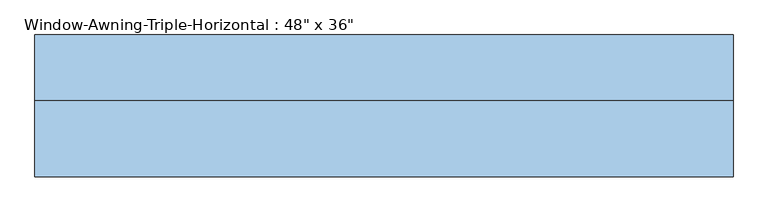
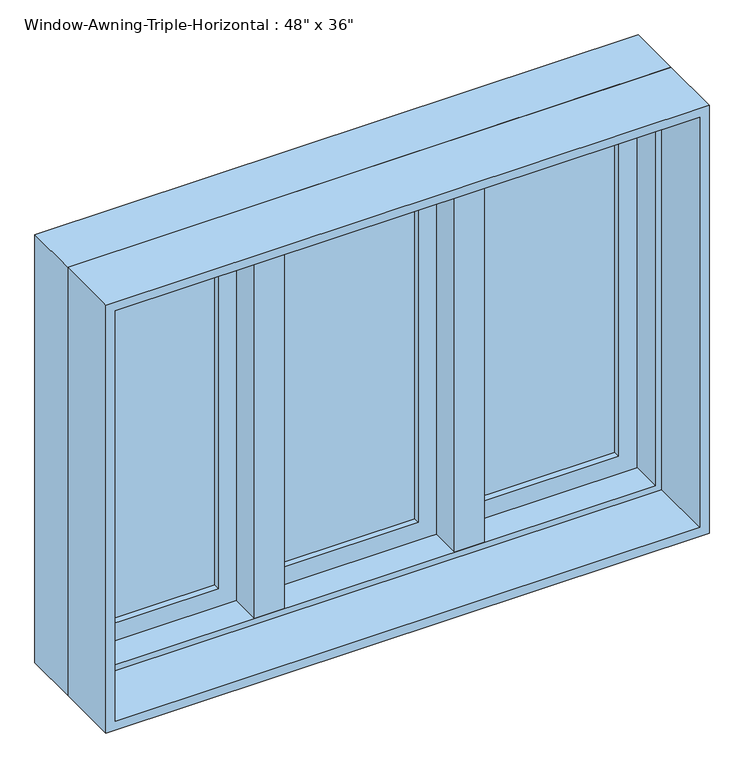
"""IFC4 building model written with IfcOpenShell, lengths in millimetres: window geometry."""

from ifc_helpers import new_model, si_unit, frame, origin, place, context, project, spatial, polyline, outline, extrude, faceted_brep, source, transform, mapped, element, save


def window_06177765(model_context):
    return source(origin(), model_context, "Body", "SolidModel", [
        faceted_brep([(577.85, 82.55, 1797.05), (577.85, 19.05, 1797.05), (-577.85, 19.05, 1797.05), (-577.85, 82.55, 1797.05), (596.9, 133.35, 1816.1), (596.9, 82.55, 1816.1), (-596.9, 82.55, 1816.1), (-596.9, 133.35, 1816.1), (609.6, 19.05, 1828.8), (609.6, 133.35, 1828.8), (-609.6, 133.35, 1828.8), (-609.6, 19.05, 1828.8), (-577.85, 19.05, 946.15), (-577.85, 82.55, 946.15), (-596.9, 82.55, 927.1), (-596.9, 133.35, 927.1), (-609.6, 133.35, 914.4), (-609.6, 19.05, 914.4), (577.85, 19.05, 946.15), (577.85, 82.55, 946.15), (596.9, 82.55, 927.1), (596.9, 133.35, 927.1), (609.6, 133.35, 914.4), (609.6, 19.05, 914.4)], [[[0, 1, 2, 3]], [[4, 5, 6, 7]], [[8, 9, 10, 11]], [[3, 2, 12, 13]], [[7, 6, 14, 15]], [[11, 10, 16, 17]], [[13, 12, 18, 19]], [[15, 14, 20, 21]], [[17, 16, 22, 23]], [[11, 17, 23, 8], [1, 18, 12, 2]], [[19, 18, 1, 0]], [[5, 20, 14, 6], [3, 13, 19, 0]], [[21, 20, 5, 4]], [[23, 22, 9, 8]], [[9, 22, 16, 10], [7, 15, 21, 4]]]),
        extrude(outline(polyline([(1828.8, -609.6), (914.4, -609.6), (914.4, 609.6), (1828.8, 609.6), (1828.8, -609.6)]), holes=[polyline([(1809.75, 590.55), (933.45, 590.55), (933.45, -590.55), (1809.75, -590.55), (1809.75, 590.55)])]), frame((0.0, -114.3, 0.0), z_axis=(0.0, 1.0, 0.0), x_axis=(0.0, 0.0, 1.0)), (0.0, 0.0, 1.0), 133.35),
        extrude(outline(polyline([(927.1, 596.9), (1816.1, 596.9), (1816.1, 211.6666667), (927.1, 211.6666667), (927.1, 596.9)]), holes=[polyline([(984.25, 268.8166667), (1758.95, 268.8166667), (1758.95, 539.75), (984.25, 539.75), (984.25, 268.8166667)])]), frame((0.0, 82.55, 0.0), z_axis=(0.0, 1.0, 0.0), x_axis=(0.0, 0.0, 1.0)), (0.0, 0.0, 1.0), 44.45),
        extrude(outline(polyline([(1816.1, -596.9), (927.1, -596.9), (927.1, -211.6666667), (1816.1, -211.6666667), (1816.1, -596.9)]), holes=[polyline([(1758.95, -268.8166667), (984.25, -268.8166667), (984.25, -539.75), (1758.95, -539.75), (1758.95, -268.8166667)])]), frame((0.0, 82.55, 0.0), z_axis=(0.0, 1.0, 0.0), x_axis=(0.0, 0.0, 1.0)), (0.0, 0.0, 1.0), 44.45),
        extrude(outline(polyline([(539.75, 114.3), (539.75, 107.95), (268.8166667, 107.95), (268.8166667, 114.3), (539.75, 114.3)])), frame((0.0, 0.0, 984.25), z_axis=(0.0, 0.0, 1.0), x_axis=(1.0, 0.0, 0.0)), (0.0, 0.0, 1.0), 774.7),
        extrude(outline(polyline([(268.8166667, 95.25), (268.8166667, 101.6), (539.75, 101.6), (539.75, 95.25), (268.8166667, 95.25)])), frame((0.0, 0.0, 984.25), z_axis=(0.0, 0.0, 1.0), x_axis=(1.0, 0.0, 0.0)), (0.0, 0.0, 1.0), 774.7),
        extrude(outline(polyline([(-268.8166667, 114.3), (-268.8166667, 107.95), (-539.75, 107.95), (-539.75, 114.3), (-268.8166667, 114.3)])), frame((0.0, 0.0, 984.25), z_axis=(0.0, 0.0, 1.0), x_axis=(1.0, 0.0, 0.0)), (0.0, 0.0, 1.0), 774.7),
        extrude(outline(polyline([(-539.75, 95.25), (-539.75, 101.6), (-268.8166667, 101.6), (-268.8166667, 95.25), (-539.75, 95.25)])), frame((0.0, 0.0, 984.25), z_axis=(0.0, 0.0, 1.0), x_axis=(1.0, 0.0, 0.0)), (0.0, 0.0, 1.0), 774.7),
        extrude(outline(polyline([(135.4666667, 114.3), (135.4666667, 107.95), (-135.4666667, 107.95), (-135.4666667, 114.3), (135.4666667, 114.3)])), frame((0.0, 0.0, 984.25), z_axis=(0.0, 0.0, 1.0), x_axis=(1.0, 0.0, 0.0)), (0.0, 0.0, 1.0), 774.7),
        extrude(outline(polyline([(-135.4666667, 95.25), (-135.4666667, 101.6), (135.4666667, 101.6), (135.4666667, 95.25), (-135.4666667, 95.25)])), frame((0.0, 0.0, 984.25), z_axis=(0.0, 0.0, 1.0), x_axis=(1.0, 0.0, 0.0)), (0.0, 0.0, 1.0), 774.7),
        extrude(outline(polyline([(927.1, 192.6166667), (1816.1, 192.6166667), (1816.1, -192.6166667), (927.1, -192.6166667), (927.1, 192.6166667)]), holes=[polyline([(984.25, -135.4666667), (1758.95, -135.4666667), (1758.95, 135.4666667), (984.25, 135.4666667), (984.25, -135.4666667)])]), frame((0.0, 82.55, 0.0), z_axis=(0.0, 1.0, 0.0), x_axis=(0.0, 0.0, 1.0)), (0.0, 0.0, 1.0), 44.45),
        faceted_brep([(192.6166667, 82.55, 1816.1), (172.1065328, 82.55, 1816.1), (172.1065328, 19.05, 1816.1), (232.1768005, 19.05, 1816.1), (232.1768005, 82.55, 1816.1), (211.6666667, 82.55, 1816.1), (211.6666667, 133.35, 1816.1), (192.6166667, 133.35, 1816.1), (192.6166667, 133.35, 927.1), (211.6666667, 133.35, 927.1), (211.6666667, 104.775, 927.1), (192.6166667, 104.775, 927.1), (192.6166667, 82.55, 1809.75), (172.1065328, 82.55, 1809.75), (192.6166667, 82.55, 1797.05), (192.6166667, 82.55, 946.15), (172.1065328, 82.55, 946.15), (172.1065328, 82.55, 1797.05), (172.1065328, 19.05, 1809.75), (172.1065328, 19.05, 946.15), (172.1065328, 19.05, 1797.05), (232.1768005, 19.05, 1809.75), (232.1768005, 19.05, 946.15), (232.1768005, 19.05, 1797.05), (232.1768005, 82.55, 1809.75), (232.1768005, 82.55, 946.15), (232.1768005, 82.55, 1797.05), (211.6666667, 82.55, 1809.75), (211.6666667, 82.55, 946.15), (211.6666667, 82.55, 1797.05), (211.6666667, 104.775, 1809.75), (211.6666667, 104.775, 1797.05), (211.6666667, 104.775, 946.15), (192.6166667, 104.775, 946.15), (192.6166667, 104.775, 1797.05), (192.6166667, 104.775, 1809.75)], [[[0, 1, 2, 3, 4, 5, 6, 7]], [[8, 9, 10, 11]], [[1, 0, 12, 13]], [[14, 15, 16, 17]], [[2, 1, 13, 18]], [[17, 16, 19, 20]], [[3, 2, 18, 21]], [[20, 19, 22, 23]], [[4, 3, 21, 24]], [[23, 22, 25, 26]], [[5, 4, 24, 27]], [[26, 25, 28, 29]], [[6, 5, 27, 30, 31, 29, 28, 32, 10, 9]], [[0, 7, 8, 11, 33, 15, 14, 34, 35, 12]], [[30, 35, 34, 31]], [[32, 33, 11, 10]], [[35, 30, 27, 24, 21, 18, 13, 12]], [[31, 34, 14, 17, 20, 23, 26, 29]], [[33, 32, 28, 25, 22, 19, 16, 15]], [[7, 6, 9, 8]]]),
        faceted_brep([(-211.6666667, 82.55, 1816.1), (-232.1768005, 82.55, 1816.1), (-232.1768005, 19.05, 1816.1), (-172.1065328, 19.05, 1816.1), (-172.1065328, 82.55, 1816.1), (-192.6166667, 82.55, 1816.1), (-192.6166667, 133.35, 1816.1), (-211.6666667, 133.35, 1816.1), (-211.6666667, 133.35, 927.1), (-192.6166667, 133.35, 927.1), (-192.6166667, 104.775, 927.1), (-211.6666667, 104.775, 927.1), (-232.1768005, 82.55, 1809.75), (-232.1768005, 19.05, 1809.75), (-232.1768005, 82.55, 1797.05), (-232.1768005, 82.55, 946.15), (-232.1768005, 19.05, 946.15), (-232.1768005, 19.05, 1797.05), (-172.1065328, 19.05, 1809.75), (-172.1065328, 19.05, 946.15), (-172.1065328, 19.05, 1797.05), (-172.1065328, 82.55, 1809.75), (-172.1065328, 82.55, 946.15), (-172.1065328, 82.55, 1797.05), (-192.6166667, 82.55, 1809.75), (-192.6166667, 104.775, 1809.75), (-192.6166667, 104.775, 1797.05), (-192.6166667, 82.55, 1797.05), (-192.6166667, 82.55, 946.15), (-192.6166667, 104.775, 946.15), (-211.6666667, 104.775, 946.15), (-211.6666667, 82.55, 946.15), (-211.6666667, 82.55, 1797.05), (-211.6666667, 104.775, 1797.05), (-211.6666667, 104.775, 1809.75), (-211.6666667, 82.55, 1809.75)], [[[0, 1, 2, 3, 4, 5, 6, 7]], [[8, 9, 10, 11]], [[2, 1, 12, 13]], [[14, 15, 16, 17]], [[3, 2, 13, 18]], [[17, 16, 19, 20]], [[4, 3, 18, 21]], [[20, 19, 22, 23]], [[6, 5, 24, 25, 26, 27, 28, 29, 10, 9]], [[0, 7, 8, 11, 30, 31, 32, 33, 34, 35]], [[25, 34, 33, 26]], [[29, 30, 11, 10]], [[34, 25, 24, 21, 18, 13, 12, 35]], [[26, 33, 32, 14, 17, 20, 23, 27]], [[30, 29, 28, 22, 19, 16, 15, 31]], [[1, 0, 35, 12]], [[15, 14, 32, 31]], [[5, 4, 21, 24]], [[28, 27, 23, 22]], [[7, 6, 9, 8]]]),
    ])


if __name__ == "__main__":
    model = new_model("IFC4")
    model_context = context("Model", 3, world=origin())
    ifc_project = project(units=[si_unit("LENGTHUNIT", "METRE", prefix="MILLI")], contexts=[model_context])
    site = spatial("IfcSite", under=ifc_project)
    building = spatial("IfcBuilding", under=site)
    placement = place(None, origin())
    window_shape = window_06177765(model_context)
    element("IfcWindow", 1, ObjectType="Window-Awning-Triple-Horizontal : 48\" x 36\"", at=placement, inside=building, context=model_context, shape_type="MappedRepresentation", body=[
        mapped(window_shape, transform((0.0, 0.0, 0.0), x_axis=(1.0, 0.0, 0.0), y_axis=(0.0, 1.0, 0.0), z_axis=(0.0, 0.0, 1.0))),
    ])
    save(model, "model.ifc")

# Revit data of these elements
# Type "Window-Awning-Triple-Horizontal : 48\" x 36\""
#   Type Mark = "24"
#   Fire Rating = "0.5h"
#   Analytic Construction = "Double glazing - domestic"
#   Window Inset [instance default] = 0' - 0"
#   Wall Thickness [instance default] = 0' - 6"
#   Muntin Width = 0' - 10.66667"
#   Visual Light Transmittance = 0.81
#   Thermal Resistance (R) = 1.8146 (h·ft²·°F)/BTU
#   Solar Heat Gain Coefficient = 0.76
#   One Third Width = 1' - 4"
#   Sash Width = 1' - 3.16667"
#   Rough Width = 4' - 0 1/2"
#   Rough Height = 3' - 0 1/2"
#   Interior Wall Closure [instance default] = 0' - 2 1/4"
#   Height = 3' - 0"
#   Heat Transfer Coefficient (U) = 0.5511 BTU/(h·ft²·°F)
#   Muntin Height = 2' - 6 1/2"
#   Frame Extension [instance default] = 0' - 0 1/4"
#   Exterior Wall Closure [instance default] = 0' - 1 1/4"
#   Extension Jamb [instance default] = 0' - 2 1/4"
#   Default Sill Height = 3' - 0"
#   Width = 4' - 0"
#   Middle Muntin Visibility = yes
#   Side Muntin Visibility = yes
#   Interior Trim Visibility [instance default] = yes
#   Exterior Trim Visibility [instance default] = yes
#   Extension Jamb Visibility [instance default] = yes
#   Muntin Pattern = Muntin Pattern_2x2 : Muntin Pattern_2x2
#   Interior Trim Material = Wood - Stained
#   Interior Trim = Trim-Window-Interior-Flat : Picture Frame
#   Interior Frame Material = Wood - Stained
#   Glass Panel Material = Glass
#   Exterior Trim Material = Clad - White
#   Exterior Trim = Trim-Window-Exterior-Flat : with Sill
#   Exterior Frame Material = Clad - White
#   Wall Closure = (empty or 0)
# Element 1 (IfcWindow, "Window-Awning-Triple-Horizontal : 48\" x 36\"")
#   Wall Thickness = 0' - 9"
#   Extension Jamb = 0' - 5 1/4"
#   Materials on its faces: "Wood - Stained", "Glass", "Clad - White"
# Materials
#   "Wood - Stained": class "Wood", colour RGB 224 178 126, transparency 0, Cost = 0
#   "Glass": class "Glass", colour RGB 0 128 192, transparency 0.75, Description = "Soda Lime Glass", Cost = 0
#   "Clad - White": class "Wood", colour RGB 242 242 238, transparency 0, Cost = 0
